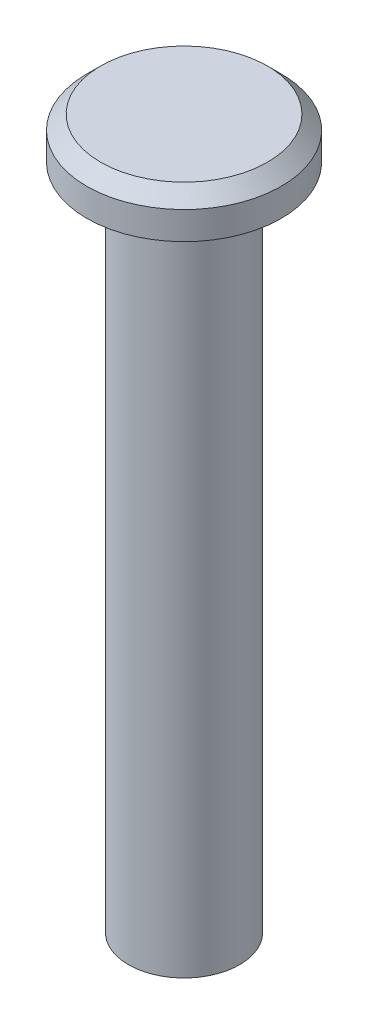
from build123d import *

# Parameters (mm, degrees)
SHANK_PROFILE_8_R      = 4
SHANK_8X48_DEPTH       = 48
HEAD_PROFILE_14_R      = 7
HEAD_14X3_DEPTH        = 3
HEAD_CHAMFER_1X45_SIZE = 1


with BuildPart() as part:
    # Shank Profile Ø8 → Shank Ø8x48 (new body)
    with BuildSketch(Plane(origin=(0, 0, 0), x_dir=(1, 0, 0), z_dir=(0, 1, 0))):
        with Locations(Location((0, 0, 0), (0, 0, 270))):
            Circle(SHANK_PROFILE_8_R)
    extrude(amount=SHANK_8X48_DEPTH)

    # Head Profile Ø14 → Head Ø14x3 (add)
    with BuildSketch(Plane(origin=(0, 48, 0), x_dir=(1, 0, 0), z_dir=(0, 1, 0))):
        with Locations(Location((0, 0, 0), (0, 0, 270))):
            Circle(HEAD_PROFILE_14_R)
    extrude(amount=HEAD_14X3_DEPTH)

    # Head Chamfer 1x45°
    head_chamfer_1x45_edges = [part.edges().sort_by_distance(p)[0] for p in [
        (0, 51, -7),
    ]]
    chamfer(head_chamfer_1x45_edges, length=HEAD_CHAMFER_1X45_SIZE)


solid = part.part
